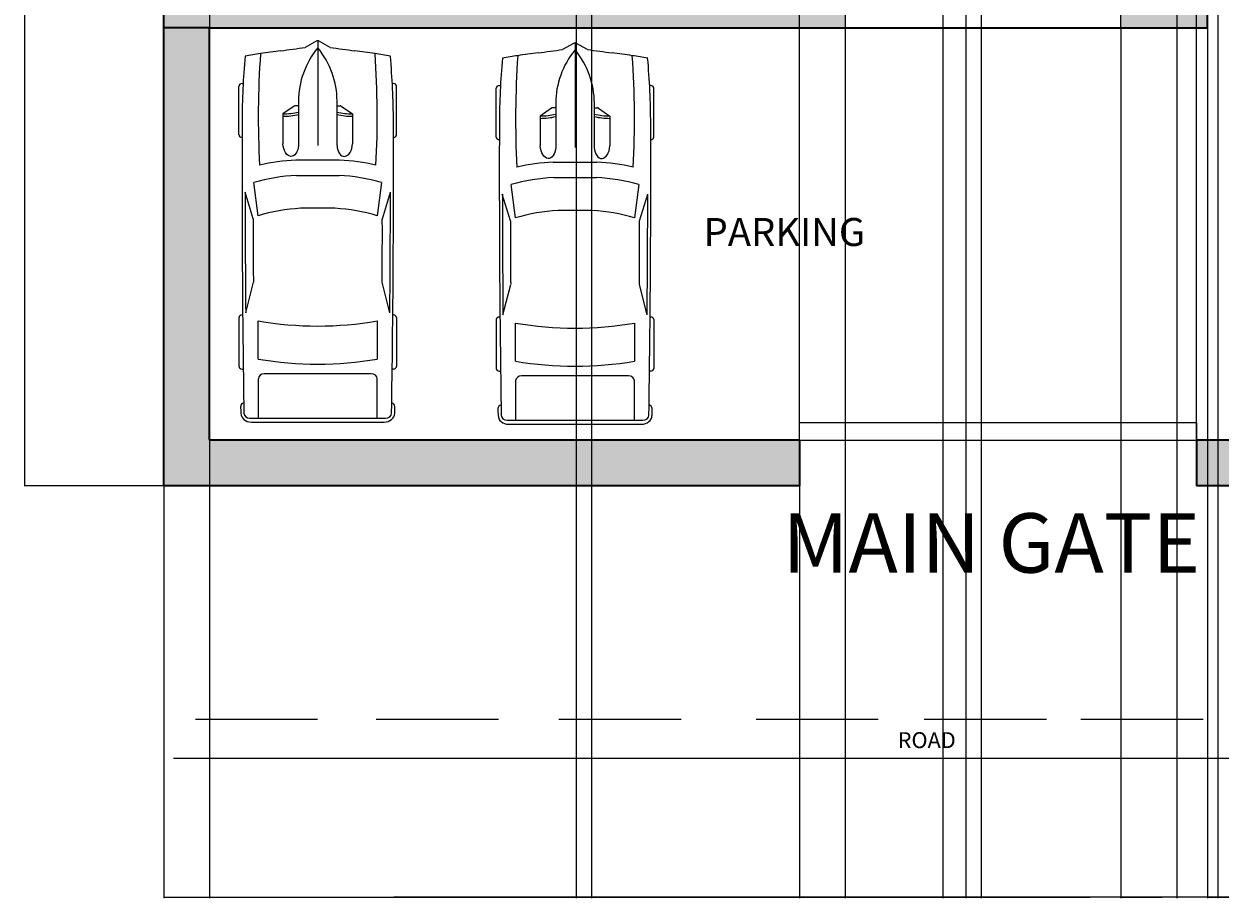
# Model space of a CAD drawing. Units: inches. Extents: x 1839 to 2285, y 722 to 1311.
# Tile 1 of 7: x 1870 to 2105, y 722 to 894. Entities that reach past the tile are written whole.
import ezdxf

# ---------------------------------------------------------------- set-up
doc = ezdxf.new("R2010")
doc.units = ezdxf.units.IN
for name, color, linetype, lineweight in [('A-ANNO-DIMS', 2, 'Continuous', 18), ('A-ANNO-TEXT', 7, 'Continuous', 18), ('A-AREA-IDEN', 7, 'Continuous', 18), ('A-DOOR', 3, 'Continuous', 25), ('A-GLAZ', 4, 'Continuous', 18), ('A-WALL', 7, 'Continuous', 35), ('C-PARK-VEHI', 8, 'Continuous', 13), ('C-ROAD', 8, 'Continuous', 18)]:
    doc.layers.add(name, color=color, linetype=linetype, lineweight=lineweight)
doc.layers.add('A-WALL-PATT', color=18, linetype='Continuous', lineweight=13, true_color=0x000000)
doc.styles.get("Standard").update_dxf_attribs({"font": 'arial.ttf'})
doc.dimstyles.get("Standard").update_dxf_attribs({"dimtxt": 0.18, "dimasz": 0.18, "dimexe": 0.18, "dimexo": 0.0625, "dimgap": 0.09, "dimtad": 0, "dimtih": 1, "dimtoh": 1, "dimdec": 4, "dimzin": 0, "dimdsep": 46, "dimtxsty": 'Standard', "dimcen": 0.09, "dimadec": 0, "dimazin": 0, "dimtfac": 1, "dimtdec": 4, "dimtofl": 0, "dimtmove": 0, "dimatfit": 3, "dimfxl": 1, "dimtolj": 1, "dimtzin": 0, "dimarcsym": 0})

# ---------------------------------------------------------------- blocks, each defined once
blk = doc.blocks.new('*U16')
for p, q in [((536, 950), (536, 936)), ((1182, 988), (568, 988)), ((1214, 950), (1214, 950)), ((2235, 810), (1899, 912)), ((3412, 904), (3030, 807)), ((3440, 942), (3440, 950)), ((3472, 988), (4087, 988)), ((4119, 950), (4119, 934)), ((1779, 801), (2195, 746)), ((4736, -851), (4736, 851)), ((4785, -832), (4785, 832)), ((3516, 746), (3994, 746)), ((4179, 670), (4179, -670)), ((4736, 746), (4242, 746)), ((820, 295), (918, 436)), ((918, 436), (1294, 436)), ((83, 156), (3, 10)), ((756, 241), (1313, 241)), ((816, 241), (816, 283)), ((1496, -274), (1496, 274)), ((1690, -267), (1690, 267)), ((2102, 216), (2102, -216)), ((4736, -267), (4736, 267)), ((0, 0), (1313, 0)), ((3, -10), (83, -156)), ((756, -241), (1313, -241)), ((816, -241), (816, -283)), ((820, -295), (918, -436)), ((918, -436), (1294, -436)), ((2195, -746), (1779, -801)), ((3994, -746), (3516, -746)), ((4242, -746), (4736, -746)), ((2235, -810), (1899, -912)), ((3412, -904), (3030, -807)), ((536, -950), (536, -936)), ((1182, -988), (568, -988)), ((1214, -950), (1214, -950)), ((3440, -942), (3440, -950)), ((3472, -988), (4087, -988)), ((4119, -950), (4119, -934))]:
    blk.add_line(p, q)
for centre, major_axis, ratio, start_param, end_param in [((6757, -699), (0, 7958), 0.842304, 1.367076, 1.39176), ((1046, -12468), (0, 13417), 0.842304, 0.00281, 0.075598), ((568, 950), (0, -37.6), 0.842304, 3.141593, 4.712389), ((1638, -268113), (0, 269063), 0.842304, -0.013397, 0.002797), ((1182, 950), (0, 37.6), 0.842304, -1.570796, 0), ((1638, -268113), (0, -269025), 0.842304, 3.133765, 3.140441), ((3472, 950), (0, -37.6), 0.842304, 3.141593, 4.712389), ((4087, 950), (0, 37.6), 0.842304, -1.570796, 0), ((4588, 910), (0, 56.4), 0.842304, -0.013017, 1.249894), ((1638, -268131), (0, 269121), 0.842304, -0.013397, -0.013017), ((4673, 851), (0, -75.2), 0.842304, 1.570796, 3.128196), ((4673, 832), (0, -133), 0.842304, 1.570796, 3.128196), ((952, -15087), (0, -15833), 0.842304, 3.096046, 3.200911), ((3436, 137), (0, 2077), 0.842304, 1.245306, 1.50788), ((2433, -93125), (0, -93935), 0.842304, 3.134049, 3.144098), ((6583, -699), (0, -7755), 0.842304, 4.528606, 4.561838), ((3414, 137), (0, -2280), 0.842304, 4.449482, 4.652344), ((3800, 71), (0, -2021), 0.842304, 4.372215, 4.640744), ((434, 0), (0, 3734), 0.842304, 4.511394, 4.913384), ((912, 0), (0, 3734), 0.842304, 4.511394, 4.913384), ((4242, 670), (0, 75.2), 0.842304, 0, 1.570796), ((-5194, 1331), (0, -6374), 0.842304, 1.385369, 1.434372), ((331, 432), (0, 696), 0.842304, 4.435146, 4.718221), ((361, 432), (0, 696), 0.842304, 4.435146, 4.718221), ((1290, 339), (161, -9), 0.603834, -1.395552, 1.581315), ((756, -1185), (0, 1427), 0.842304, 0, 0.590319), ((832, 283), (0, 18.8), 0.842304, 0.879714, 1.570796), ((16, 0), (0, -18.8), 0.842304, 4.131459, 5.293319), ((756, 1185), (0, 1427), 0.842304, 2.551274, 3.141593), ((-5194, -1331), (0, 6374), 0.842304, -1.434372, -1.385369), ((832, -283), (0, -18.8), 0.842304, 4.712389, 5.403472), ((331, -432), (0, -696), 0.842304, 1.564964, 1.848039), ((361, -432), (0, -696), 0.842304, 1.564964, 1.848039), ((3414, -137), (0, -2280), 0.842304, -1.510751, -1.307889), ((3436, -137), (0, -2077), 0.842304, -1.50788, -1.245306), ((3800, -71), (0, -2021), 0.842304, -1.499151, -1.230623), ((6583, 699), (0, 7755), 0.842304, 1.721348, 1.754579), ((6757, 699), (0, 7958), 0.842304, 1.749832, 1.774517), ((952, 15087), (0, -15833), 0.842304, -0.059319, 0.045547), ((4242, -670), (0, -75.2), 0.842304, 4.712389, 6.283185), ((2433, 93125), (0, -93935), 0.842304, -0.002505, 0.007544), ((4673, -851), (0, 75.2), 0.842304, 3.15499, 4.712389), ((4673, -832), (0, -133), 0.842304, 0.013397, 1.570796), ((1046, 12468), (0, -13417), 0.842304, -0.075598, -0.00281), ((568, -950), (0, 37.6), 0.842304, 1.570796, 3.141593), ((1638, 268113), (0, 269063), 0.842304, 3.138796, 3.15499), ((1182, -950), (0, -37.6), 0.842304, 0, 1.570796), ((1638, 268113), (0, -269025), 0.842304, 0.001152, 0.007828), ((3472, -950), (0, -37.6), 0.842304, -1.570796, 0), ((4087, -950), (0, 37.6), 0.842304, 3.141593, 4.712389), ((4588, -910), (0, -56.4), 0.842304, -1.249894, 0.013017), ((1638, 268131), (0, 269121), 0.842304, 3.15461, 3.15499)]:
    blk.add_ellipse(centre, major_axis=major_axis, ratio=ratio, start_param=start_param, end_param=end_param)
at = {"extrusion": (0, 0, -1)}
blk.add_ellipse((1290, -339), major_axis=(161, 9), ratio=0.603834, start_param=-1.395552, end_param=1.581315, dxfattribs=at)
blk = doc.blocks.new('*D41')
at = {"layer": 'A-ANNO-DIMS', "color": 0, "lineweight": -2, "transparency": 16777216}
for p, q in [((1897.68, 803.27), (1897.68, 722.34)), ((2257.68, 803.27), (2257.68, 722.34)), ((1897.86, 722.52), (2077.39, 722.52)), ((2257.5, 722.52), (2077.97, 722.52))]:
    blk.add_line(p, q, dxfattribs=at)
at = {"layer": 'A-ANNO-DIMS', "color": 0, "transparency": 16777216}
for points in [[(1897.86, 722.55), (1897.86, 722.49), (1897.68, 722.52)], [(2257.5, 722.55), (2257.5, 722.49), (2257.68, 722.52)]]:
    blk.add_solid(points, dxfattribs=at)
at = {"layer": 'Defpoints', "color": 0, "transparency": 16777216}
for p in [(1897.68, 803.33), (2257.68, 803.33), (2257.68, 722.52)]:
    blk.add_point(p, dxfattribs=at)
at = {"layer": 'A-ANNO-DIMS', "color": 0, "transparency": 16777216, "insert": (2077.68, 722.52), "char_height": 0.18, "attachment_point": 5}
blk.add_mtext('\\A1;360', dxfattribs=at)
blk = doc.blocks.new('*D42')
at = {"layer": 'A-ANNO-DIMS', "color": 0, "lineweight": -2, "transparency": 16777216}
for p, q in [((1897.61, 1283.33), (1870.25, 1283.33)), ((1870.43, 1283.15), (1870.43, 1043.51)), ((1870.43, 803.51), (1870.43, 1043.15)), ((1897.61, 803.33), (1870.25, 803.33))]:
    blk.add_line(p, q, dxfattribs=at)
at = {"layer": 'A-ANNO-DIMS', "color": 0, "transparency": 16777216}
for points in [[(1870.4, 1283.15), (1870.46, 1283.15), (1870.43, 1283.33)], [(1870.4, 803.51), (1870.46, 803.51), (1870.43, 803.33)]]:
    blk.add_solid(points, dxfattribs=at)
at = {"layer": 'Defpoints', "color": 0, "transparency": 16777216}
for p in [(1870.43, 1283.33), (1897.68, 1283.33), (1897.68, 803.33)]:
    blk.add_point(p, dxfattribs=at)
at = {"layer": 'A-ANNO-DIMS', "color": 0, "transparency": 16777216, "insert": (1870.43, 1043.33), "char_height": 0.18, "attachment_point": 5}
blk.add_mtext('\\A1;480', dxfattribs=at)
blk = doc.blocks.new('*D43')
at = {"layer": 'A-ANNO-DIMS', "color": 0, "lineweight": -2, "transparency": 16777216}
for p, q in [((2050.68, 1145.27), (2050.68, 722.34)), ((1906.68, 1142.27), (1906.68, 722.34)), ((1906.86, 722.52), (1978.4, 722.52)), ((2050.5, 722.52), (1978.96, 722.52))]:
    blk.add_line(p, q, dxfattribs=at)
at = {"layer": 'A-ANNO-DIMS', "color": 0, "transparency": 16777216}
for points in [[(1906.86, 722.55), (1906.86, 722.49), (1906.68, 722.52)], [(2050.5, 722.55), (2050.5, 722.49), (2050.68, 722.52)]]:
    blk.add_solid(points, dxfattribs=at)
at = {"layer": 'Defpoints', "color": 0, "transparency": 16777216}
for p in [(2050.68, 1145.33), (1906.68, 1142.33), (2050.68, 722.52)]:
    blk.add_point(p, dxfattribs=at)
at = {"layer": 'A-ANNO-DIMS', "color": 0, "transparency": 16777216, "insert": (1978.68, 722.52), "char_height": 0.18, "attachment_point": 5}
blk.add_mtext('\\A1;144', dxfattribs=at)
blk = doc.blocks.new('*D44')
at = {"layer": 'A-ANNO-DIMS', "color": 0, "lineweight": -2, "transparency": 16777216}
for p, q in [((2055.18, 1137.77), (2055.18, 722.34)), ((2104.68, 1137.77), (2104.68, 722.34)), ((2055.36, 722.52), (2079.6, 722.52)), ((2104.5, 722.52), (2080.26, 722.52))]:
    blk.add_line(p, q, dxfattribs=at)
at = {"layer": 'A-ANNO-DIMS', "color": 0, "transparency": 16777216}
for points in [[(2055.36, 722.55), (2055.36, 722.49), (2055.18, 722.52)], [(2104.5, 722.55), (2104.5, 722.49), (2104.68, 722.52)]]:
    blk.add_solid(points, dxfattribs=at)
at = {"layer": 'Defpoints', "color": 0, "transparency": 16777216}
for p in [(2055.18, 1137.83), (2104.68, 1137.83), (2104.68, 722.52)]:
    blk.add_point(p, dxfattribs=at)
at = {"layer": 'A-ANNO-DIMS', "color": 0, "transparency": 16777216, "insert": (2079.93, 722.52), "char_height": 0.18, "attachment_point": 5}
blk.add_mtext('\\A1;49.5', dxfattribs=at)
blk = doc.blocks.new('*D50')
at = {"layer": 'A-ANNO-DIMS', "color": 0, "lineweight": -2, "transparency": 16777216}
for p, q in [((2145.57, 893.33), (2285.11, 893.33)), ((2284.93, 893.15), (2284.93, 853.01)), ((2284.93, 812.51), (2284.93, 852.65)), ((1906.74, 812.33), (2285.11, 812.33))]:
    blk.add_line(p, q, dxfattribs=at)
at = {"layer": 'A-ANNO-DIMS', "color": 0, "transparency": 16777216}
for points in [[(2284.9, 893.15), (2284.96, 893.15), (2284.93, 893.33)], [(2284.9, 812.51), (2284.96, 812.51), (2284.93, 812.33)]]:
    blk.add_solid(points, dxfattribs=at)
at = {"layer": 'Defpoints', "color": 0, "transparency": 16777216}
for p in [(2145.5, 893.33), (2284.93, 893.33), (1906.68, 812.33)]:
    blk.add_point(p, dxfattribs=at)
at = {"layer": 'A-ANNO-DIMS', "color": 0, "transparency": 16777216, "insert": (2284.93, 852.83), "char_height": 0.18, "attachment_point": 5}
blk.add_mtext('\\A1;81', dxfattribs=at)
blk = doc.blocks.new('*D51')
at = {"layer": 'A-ANNO-DIMS', "color": 0, "lineweight": -2, "transparency": 16777216}
for p, q in [((1906.68, 897.77), (1906.68, 722.34)), ((1978.68, 897.77), (1978.68, 722.34)), ((1906.86, 722.52), (1942.46, 722.52)), ((1978.5, 722.52), (1942.89, 722.52))]:
    blk.add_line(p, q, dxfattribs=at)
at = {"layer": 'A-ANNO-DIMS', "color": 0, "transparency": 16777216}
for points in [[(1906.86, 722.55), (1906.86, 722.49), (1906.68, 722.52)], [(1978.5, 722.55), (1978.5, 722.49), (1978.68, 722.52)]]:
    blk.add_solid(points, dxfattribs=at)
at = {"layer": 'Defpoints', "color": 0, "transparency": 16777216}
for p in [(1906.68, 897.83), (1978.68, 897.83), (1978.68, 722.52)]:
    blk.add_point(p, dxfattribs=at)
at = {"layer": 'A-ANNO-DIMS', "color": 0, "transparency": 16777216, "insert": (1942.68, 722.52), "char_height": 0.18, "attachment_point": 5}
blk.add_mtext('\\A1;72', dxfattribs=at)
blk = doc.blocks.new('*D52')
at = {"layer": 'A-ANNO-DIMS', "color": 0, "lineweight": -2, "transparency": 16777216}
for p, q in [((1981.68, 1013.27), (1981.68, 722.34)), ((2096.66, 1013.27), (2096.66, 722.34)), ((1981.86, 722.52), (2038.72, 722.52)), ((2096.48, 722.52), (2039.63, 722.52))]:
    blk.add_line(p, q, dxfattribs=at)
at = {"layer": 'A-ANNO-DIMS', "color": 0, "transparency": 16777216}
for points in [[(1981.86, 722.55), (1981.86, 722.49), (1981.68, 722.52)], [(2096.48, 722.55), (2096.48, 722.49), (2096.66, 722.52)]]:
    blk.add_solid(points, dxfattribs=at)
at = {"layer": 'Defpoints', "color": 0, "transparency": 16777216}
for p in [(1981.68, 1013.33), (2096.66, 1013.33), (2096.66, 722.52)]:
    blk.add_point(p, dxfattribs=at)
at = {"layer": 'A-ANNO-DIMS', "color": 0, "transparency": 16777216, "insert": (2039.17, 722.52), "char_height": 0.18, "attachment_point": 5}
blk.add_mtext('\\A1;114.99', dxfattribs=at)
blk = doc.blocks.new('*D55')
at = {"layer": 'A-ANNO-DIMS', "color": 0, "lineweight": -2, "transparency": 16777216}
for p, q in [((2022.5, 812.39), (2022.5, 1310.76)), ((2100.5, 812.39), (2100.5, 1310.76)), ((2022.68, 1310.58), (2061.29, 1310.58)), ((2100.32, 1310.58), (2061.72, 1310.58))]:
    blk.add_line(p, q, dxfattribs=at)
at = {"layer": 'A-ANNO-DIMS', "color": 0, "transparency": 16777216}
for points in [[(2022.68, 1310.61), (2022.68, 1310.55), (2022.5, 1310.58)], [(2100.32, 1310.61), (2100.32, 1310.55), (2100.5, 1310.58)]]:
    blk.add_solid(points, dxfattribs=at)
at = {"layer": 'Defpoints', "color": 0, "transparency": 16777216}
for p in [(2100.5, 1310.58), (2022.5, 812.33), (2100.5, 812.33)]:
    blk.add_point(p, dxfattribs=at)
at = {"layer": 'A-ANNO-DIMS', "color": 0, "transparency": 16777216, "insert": (2061.5, 1310.58), "char_height": 0.18, "attachment_point": 5}
blk.add_mtext('\\A1;78', dxfattribs=at)
blk = doc.blocks.new('*D58')
at = {"layer": 'A-ANNO-DIMS', "color": 0, "lineweight": -2, "transparency": 16777216}
for p, q in [((2102.66, 893.27), (2102.66, 722.34)), ((2138.66, 893.27), (2138.66, 722.34)), ((2102.84, 722.52), (2120.45, 722.52)), ((2138.48, 722.52), (2120.88, 722.52))]:
    blk.add_line(p, q, dxfattribs=at)
at = {"layer": 'A-ANNO-DIMS', "color": 0, "transparency": 16777216}
for points in [[(2102.84, 722.55), (2102.84, 722.49), (2102.66, 722.52)], [(2138.48, 722.55), (2138.48, 722.49), (2138.66, 722.52)]]:
    blk.add_solid(points, dxfattribs=at)
at = {"layer": 'Defpoints', "color": 0, "transparency": 16777216}
for p in [(2102.66, 893.33), (2138.66, 893.33), (2138.66, 722.52)]:
    blk.add_point(p, dxfattribs=at)
at = {"layer": 'A-ANNO-DIMS', "color": 0, "transparency": 16777216, "insert": (2120.66, 722.52), "char_height": 0.18, "attachment_point": 5}
blk.add_mtext('\\A1;36', dxfattribs=at)
blk = doc.blocks.new('*D65')
at = {"layer": 'A-ANNO-DIMS', "color": 0, "lineweight": -2, "transparency": 16777216}
for p, q in [((1906.68, 812.27), (1906.68, 722.34)), ((2022.5, 812.27), (2022.5, 722.34)), ((1906.86, 722.52), (1964.14, 722.52)), ((2022.32, 722.52), (1965.05, 722.52))]:
    blk.add_line(p, q, dxfattribs=at)
at = {"layer": 'A-ANNO-DIMS', "color": 0, "transparency": 16777216}
for points in [[(1906.86, 722.55), (1906.86, 722.49), (1906.68, 722.52)], [(2022.32, 722.55), (2022.32, 722.49), (2022.5, 722.52)]]:
    blk.add_solid(points, dxfattribs=at)
at = {"layer": 'Defpoints', "color": 0, "transparency": 16777216}
for p in [(1906.68, 812.33), (2022.5, 812.33), (2022.5, 722.52)]:
    blk.add_point(p, dxfattribs=at)
at = {"layer": 'A-ANNO-DIMS', "color": 0, "transparency": 16777216, "insert": (1964.59, 722.52), "char_height": 0.18, "attachment_point": 5}
blk.add_mtext('\\A1;115.83', dxfattribs=at)
blk = doc.blocks.new('*D67')
at = {"layer": 'A-ANNO-DIMS', "color": 0, "lineweight": -2, "transparency": 16777216}
for p, q in [((2031.47, 893.27), (2031.47, 722.34)), ((2085.61, 893.27), (2085.61, 722.34)), ((2031.65, 722.52), (2058.15, 722.52)), ((2085.43, 722.52), (2058.93, 722.52))]:
    blk.add_line(p, q, dxfattribs=at)
at = {"layer": 'A-ANNO-DIMS', "color": 0, "transparency": 16777216}
for points in [[(2031.65, 722.55), (2031.65, 722.49), (2031.47, 722.52)], [(2085.43, 722.55), (2085.43, 722.49), (2085.61, 722.52)]]:
    blk.add_solid(points, dxfattribs=at)
at = {"layer": 'Defpoints', "color": 0, "transparency": 16777216}
for p in [(2031.47, 893.33), (2085.61, 893.33), (2085.61, 722.52)]:
    blk.add_point(p, dxfattribs=at)
at = {"layer": 'A-ANNO-DIMS', "color": 0, "transparency": 16777216, "insert": (2058.54, 722.52), "char_height": 0.18, "attachment_point": 5}
blk.add_mtext('\\A1;54.15', dxfattribs=at)
blk = doc.blocks.new('*D68')
at = {"layer": 'A-ANNO-DIMS', "color": 0, "lineweight": -2, "transparency": 16777216}
for p, q in [((2085.61, 893.27), (2085.61, 722.34)), ((2102.66, 893.27), (2102.66, 722.34)), ((2085.79, 722.52), (2093.75, 722.52)), ((2102.48, 722.52), (2094.52, 722.52))]:
    blk.add_line(p, q, dxfattribs=at)
at = {"layer": 'A-ANNO-DIMS', "color": 0, "transparency": 16777216}
for points in [[(2085.79, 722.55), (2085.79, 722.49), (2085.61, 722.52)], [(2102.48, 722.55), (2102.48, 722.49), (2102.66, 722.52)]]:
    blk.add_solid(points, dxfattribs=at)
at = {"layer": 'Defpoints', "color": 0, "transparency": 16777216}
for p in [(2085.61, 893.33), (2102.66, 893.33), (2102.66, 722.52)]:
    blk.add_point(p, dxfattribs=at)
at = {"layer": 'A-ANNO-DIMS', "color": 0, "transparency": 16777216, "insert": (2094.14, 722.52), "char_height": 0.18, "attachment_point": 5}
blk.add_mtext('\\A1;17.05', dxfattribs=at)
blk = doc.blocks.new('*D71')
at = {"layer": 'A-ANNO-DIMS', "color": 0, "lineweight": -2, "transparency": 16777216}
for p, q in [((1978.68, 897.77), (1978.68, 722.34)), ((1981.68, 897.77), (1981.68, 722.34)), ((1978.86, 722.52), (1980.03, 722.52)), ((1981.5, 722.52), (1980.33, 722.52))]:
    blk.add_line(p, q, dxfattribs=at)
at = {"layer": 'A-ANNO-DIMS', "color": 0, "transparency": 16777216}
for points in [[(1978.86, 722.55), (1978.86, 722.49), (1978.68, 722.52)], [(1981.5, 722.55), (1981.5, 722.49), (1981.68, 722.52)]]:
    blk.add_solid(points, dxfattribs=at)
at = {"layer": 'Defpoints', "color": 0, "transparency": 16777216}
for p in [(1978.68, 897.83), (1981.68, 897.83), (1981.68, 722.52)]:
    blk.add_point(p, dxfattribs=at)
at = {"layer": 'A-ANNO-DIMS', "color": 0, "transparency": 16777216, "insert": (1980.18, 722.52), "char_height": 0.18, "attachment_point": 5}
blk.add_mtext('\\A1;3', dxfattribs=at)
blk = doc.blocks.new('*D84')
at = {"layer": 'A-ANNO-DIMS', "color": 0, "lineweight": -2, "transparency": 16777216}
for p, q in [((2055.18, 1218.77), (2055.18, 722.34)), ((2058.18, 1218.77), (2058.18, 722.34)), ((2055.36, 722.52), (2056.53, 722.52)), ((2058, 722.52), (2056.83, 722.52))]:
    blk.add_line(p, q, dxfattribs=at)
at = {"layer": 'A-ANNO-DIMS', "color": 0, "transparency": 16777216}
for points in [[(2055.36, 722.55), (2055.36, 722.49), (2055.18, 722.52)], [(2058, 722.55), (2058, 722.49), (2058.18, 722.52)]]:
    blk.add_solid(points, dxfattribs=at)
at = {"layer": 'Defpoints', "color": 0, "transparency": 16777216}
for p in [(2055.18, 1218.83), (2058.18, 1218.83), (2058.18, 722.52)]:
    blk.add_point(p, dxfattribs=at)
at = {"layer": 'A-ANNO-DIMS', "color": 0, "transparency": 16777216, "insert": (2056.68, 722.52), "char_height": 0.18, "attachment_point": 5}
blk.add_mtext('\\A1;3', dxfattribs=at)

msp = doc.modelspace()

# ---------------------------------------------------------------- hatches: boundary and pattern name
at = {"layer": 'A-WALL-PATT'}
h = msp.add_hatch(color=256, dxfattribs=at)
h.dxf.hatch_style = 1
h.paths.add_polyline_path([(1906.6771, 1274.3314), (1942.6771, 1274.3314), (1942.6771, 1283.3314), (1897.6771, 1283.3314), (1897.6771, 968.2107), (1906.6771, 968.2107), (1906.6771, 1013.3314), (1939.6771, 1013.3314), (1939.6771, 1017.8314), (1906.6771, 1017.8314), (1906.6771, 1137.8314), (2050.6771, 1137.8314), (2050.6771, 1142.3314), (1906.6771, 1142.3314)])
h.paths.add_polyline_path([(2064.0508, 1283.3314), (1978.6771, 1283.3314), (1978.6771, 1274.3314), (2050.6771, 1274.3314), (2050.6771, 1184.3314), (2055.1771, 1184.3314), (2055.1771, 1214.3314), (2058.1771, 1214.3314), (2058.1771, 1218.8314), (2055.1771, 1218.8314), (2055.1771, 1274.3314), (2064.0508, 1274.3314)])
h.paths.add_polyline_path([(2182.6416, 1283.3314), (2088.0508, 1283.3314), (2088.0508, 1274.3314), (2104.6771, 1274.3314), (2104.6771, 1218.8314), (2094.1771, 1218.8314), (2094.1771, 1214.3314), (2104.6771, 1214.3314), (2104.6771, 1184.3314), (2109.1771, 1184.3314), (2109.1771, 1274.3314), (2182.6416, 1274.3314)])
h.paths.add_polyline_path([(2257.6771, 1283.3314), (2218.6416, 1283.3314), (2218.6416, 1274.3314), (2248.6771, 1274.3314), (2248.6771, 1142.3314), (2186.4004, 1142.3314), (2109.1771, 1142.3314), (2109.1771, 1137.8314), (2248.6771, 1137.8314), (2248.6771, 1094.9086), (2257.6771, 1094.9086)])
h.paths.add_polyline_path([(2257.6771, 1058.9086), (2248.6771, 1058.9086), (2248.6771, 1017.8314), (2160.1771, 1017.8314), (2160.1771, 939.8314), (2164.6771, 939.8314), (2164.6771, 1013.3314), (2248.6771, 1013.3314), (2248.6771, 977.3314), (2248.6771, 950.4862), (2257.6771, 950.4862)])
h.paths.add_polyline_path([(2257.6771, 893.3314), (2248.6771, 893.3314), (2248.6771, 850.1143), (2190.4862, 850.1143), (2190.4862, 845.6143), (2248.6771, 845.6143), (2248.6771, 812.3314), (2100.5038, 812.3314), (2100.5038, 803.3314), (2257.6771, 803.3314)])
h.paths.add_polyline_path([(2257.6771, 926.4862), (2248.6771, 926.4862), (2248.6771, 897.8314), (2141.6642, 897.8314), (2141.6642, 893.3314), (2145.5038, 893.3314), (2145.5038, 812.3314), (2147.5038, 812.3314), (2147.5038, 845.6143), (2153.9854, 845.6143), (2153.9854, 850.1143), (2147.5038, 850.1143), (2147.5038, 893.3314), (2248.6771, 893.3314), (2257.6771, 893.3314)])
h.paths.add_polyline_path([(1906.6771, 893.3314), (1897.6771, 893.3314), (1897.6771, 803.3314), (2022.5038, 803.3314), (2022.5038, 812.3314), (1906.6771, 812.3314)])
h.paths.add_polyline_path([(2031.4676, 897.8314), (1981.6771, 897.8314), (1981.6771, 1013.3314), (2024.6642, 1013.3314), (2024.6642, 1017.8314), (1975.6771, 1017.8314), (1975.6771, 1013.3314), (1978.6771, 1013.3314), (1978.6771, 897.8314), (1906.6771, 897.8314), (1906.6771, 932.2107), (1897.6771, 932.2107), (1897.6771, 893.3314), (1906.6771, 893.3314), (2031.4676, 893.3314)])
h.paths.add_polyline_path([(2099.6642, 1017.8314), (2096.6642, 1017.8314), (2084.1956, 1017.8314), (2084.1956, 1013.3314), (2096.6642, 1013.3314), (2096.6642, 897.8314), (2085.6129, 897.8314), (2085.6129, 893.3314), (2102.6642, 893.3314), (2102.6642, 897.8314), (2099.6642, 897.8314)])

# ---------------------------------------------------------------- linework, layer by layer
at = {"layer": 'A-DOOR'}
for p, q in [((2022.5038, 812.3314), (2022.5038, 815.7735)), ((2022.5038, 815.7735), (2100.5038, 815.7735)), ((2100.5038, 815.7735), (2100.5038, 812.3314))]:
    msp.add_line(p, q, dxfattribs=at)
at = {"layer": 'A-GLAZ'}
for p, q in [((2031.4676, 897.8314), (2031.4676, 893.3314)), ((2085.6129, 893.3314), (2085.6129, 897.8314)), ((2031.4676, 893.3314), (2085.6129, 893.3314))]:
    msp.add_line(p, q, dxfattribs=at)
at = {"layer": 'A-WALL'}
for p, q in [((2102.6642, 893.3314), (2102.6642, 897.8314)), ((1906.6771, 893.3314), (1897.6771, 893.3314)), ((1906.6771, 812.3314), (1906.6771, 893.3314)), ((1906.6771, 893.3314), (2102.6642, 893.3314)), ((2022.5038, 812.3314), (1906.6771, 812.3314)), ((2022.5038, 812.3314), (2022.5038, 803.3314)), ((2248.6771, 812.3314), (2100.5038, 812.3314)), ((2100.5038, 812.3314), (2100.5038, 803.3314))]:
    msp.add_line(p, q, dxfattribs=at)
msp.add_lwpolyline([(2022.5038, 803.3314), (1897.6771, 803.3314), (1897.6771, 1283.3314), (2257.6771, 1283.3314), (2257.6771, 803.3314), (2100.5038, 803.3314)], dxfattribs=at)
at = {"layer": 'C-ROAD'}
for p, q in [((1903.9078, 757.4754), (1927.9078, 757.4754)), ((1939.4272, 757.4754), (1963.4272, 757.4754)), ((1975.276, 757.4754), (1999.276, 757.4754)), ((2014.0019, 757.4754), (2038.0019, 757.4754)), ((2047.0393, 757.4754), (2071.0393, 757.4754)), ((2077.7989, 757.4754), (2101.7989, 757.4754)), ((2254.1419, 749.766), (1899.596, 749.766))]:
    msp.add_line(p, q, dxfattribs=at)

# ---------------------------------------------------------------- block references
at = {"layer": 'C-PARK-VEHI', "xscale": 0.0156585448006182, "yscale": 0.0156585448006182, "zscale": 0.0156585448006182, "rotation": 270}
for p in [(1927.9258, 890.7749), (1978.4541, 890.3627)]:
    msp.add_blockref('*U16', p, dxfattribs=at)

# ---------------------------------------------------------------- texts
at = {"layer": 'A-ANNO-TEXT'}
for s, height, p in [('MAIN GATE ', 11.68078, (2019.2178, 786.2678)), ('ROAD ', 3.12803, (2041.8115, 751.8016))]:
    msp.add_text(s, height=height, dxfattribs=at).set_placement(p)
at = {"layer": 'A-AREA-IDEN'}
msp.add_text('PARKING ', height=5.50379, dxfattribs=at).set_placement((2003.699, 850.4463))

# ---------------------------------------------------------------- dimensions: what is measured, and where the dimension line sits
at = {"layer": 'A-ANNO-DIMS'}
for base, p1, p2, override, picture, middle in [((2100.5038, 1310.5814), (2022.5038, 812.3314), (2100.5038, 812.3314), {"dimdec": 0, "dimlfac": 1, "dimrnd": 0, "dimzin": 0, "dimdsep": 46, "dimlunit": 2}, '*D55', (2061.5038, 1310.5814)), ((2058.1771, 722.516), (2055.1771, 1218.8314), (2058.1771, 1218.8314), {"dimdec": 0, "dimlfac": 1, "dimrnd": 0, "dimzin": 0, "dimdsep": 46, "dimlunit": 2}, '*D84', (2056.6771, 722.516)), ((2050.6771, 722.516), (1906.6771, 1142.3314), (2050.6771, 1145.3314), {"dimdec": 0, "dimlfac": 1, "dimrnd": 0, "dimzin": 0, "dimdsep": 46, "dimlunit": 2}, '*D43', (1978.6771, 722.516)), ((2104.6771, 722.516), (2055.1771, 1137.8314), (2104.6771, 1137.8314), {"dimdec": 1, "dimlfac": 1, "dimrnd": 0, "dimzin": 0, "dimdsep": 46, "dimlunit": 2}, '*D44', (2079.9271, 722.516)), ((2096.6642, 722.516), (1981.6771, 1013.3314), (2096.6642, 1013.3314), {"dimdec": 2, "dimlfac": 1, "dimrnd": 0, "dimzin": 0, "dimdsep": 46, "dimlunit": 2}, '*D52', (2039.1706, 722.516)), ((1978.6771, 722.516), (1906.6771, 897.8314), (1978.6771, 897.8314), {"dimdec": 0, "dimlfac": 1, "dimrnd": 0, "dimzin": 0, "dimdsep": 46, "dimlunit": 2}, '*D51', (1942.6771, 722.516)), ((1981.6771, 722.516), (1978.6771, 897.8314), (1981.6771, 897.8314), {"dimdec": 0, "dimlfac": 1, "dimrnd": 0, "dimzin": 0, "dimdsep": 46, "dimlunit": 2}, '*D71', (1980.1771, 722.516)), ((2085.6129, 722.516), (2031.4676, 893.3314), (2085.6129, 893.3314), {"dimdec": 2, "dimlfac": 1, "dimrnd": 0, "dimzin": 0, "dimdsep": 46, "dimlunit": 2}, '*D67', (2058.5402, 722.516)), ((2102.6642, 722.516), (2085.6129, 893.3314), (2102.6642, 893.3314), {"dimdec": 2, "dimlfac": 1, "dimrnd": 0, "dimzin": 0, "dimdsep": 46, "dimlunit": 2}, '*D68', (2094.1385, 722.516)), ((2138.6642, 722.516), (2102.6642, 893.3314), (2138.6642, 893.3314), {"dimdec": 0, "dimlfac": 1, "dimrnd": 0, "dimzin": 0, "dimdsep": 46, "dimlunit": 2}, '*D58', (2120.6642, 722.516)), ((2022.5038, 722.516), (1906.6771, 812.3314), (2022.5038, 812.3314), {"dimdec": 2, "dimlfac": 1, "dimrnd": 0, "dimzin": 0, "dimdsep": 46, "dimlunit": 2}, '*D65', (1964.5905, 722.516)), ((2257.6771, 722.516), (1897.6771, 803.3314), (2257.6771, 803.3314), {"dimdec": 0, "dimlfac": 1, "dimrnd": 0, "dimzin": 0, "dimdsep": 46, "dimlunit": 2}, '*D41', (2077.6771, 722.516))]:
    dim = msp.add_linear_dim(base=base, p1=p1, p2=p2, dimstyle='Standard', override=override, dxfattribs=at)
    dim.commit()
    dim.dimension.update_dxf_attribs({"geometry": picture, "text_midpoint": middle})
for base, p1, p2, picture, middle in [((1870.4271, 1283.3314), (1897.6771, 803.3314), (1897.6771, 1283.3314), '*D42', (1870.4271, 1043.3314)), ((2284.9271, 893.3314), (1906.6771, 812.3314), (2145.5038, 893.3314), '*D50', (2284.9271, 852.8314))]:
    dim = msp.add_linear_dim(base=base, p1=p1, p2=p2, angle=90, dimstyle='Standard', override={"dimdec": 0, "dimlfac": 1, "dimrnd": 0, "dimzin": 0, "dimdsep": 46, "dimlunit": 2}, dxfattribs=at)
    dim.commit()
    dim.dimension.update_dxf_attribs({"geometry": picture, "text_midpoint": middle})

doc.saveas('drawing.dxf')
